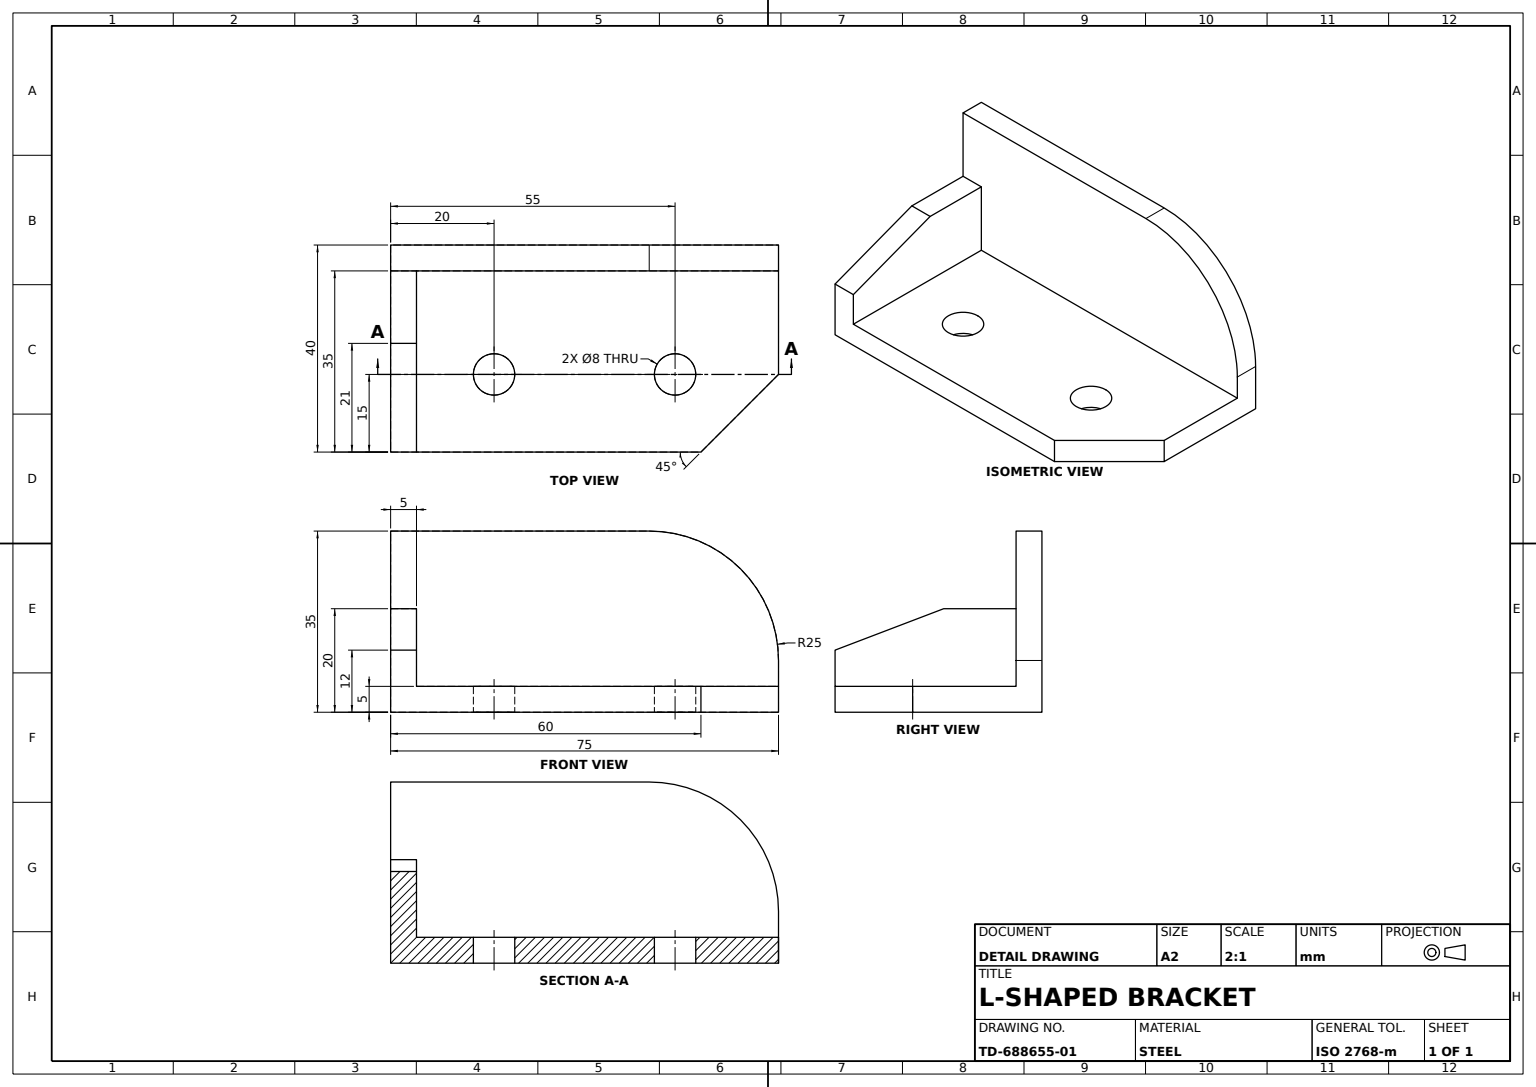
from build123d import *

# Parameters (mm, degrees)
BASE_PLATE_SKETCH_R           = 4
BASE_PLATE_DEPTH              = 5
SIDE_WALL_SKETCH_W            = 5
SIDE_WALL_SKETCH_H            = 40
SIDE_WALL_DEPTH               = 20
SIDE_WALL_TAPER_CUT_DEPTH     = 20
BACK_WALL_SKETCH_W            = 75
BACK_WALL_SKETCH_H            = 5
BACK_WALL_DEPTH               = 30
BACK_WALL_CORNER_RADIUS_DEPTH = 30


with BuildPart() as part:
    # Base Plate Sketch → Base Plate (new body)
    with BuildSketch(Plane(origin=(0, 0, 0), x_dir=(1, 0, 0), z_dir=(0, 1, 0))):
        Polygon((0, 0), (75, 0), (75, -25), (60, -40), (0, -40), align=None)
        with Locations(Location((20, -25, 0), (0, 0, 270))):
            Circle(BASE_PLATE_SKETCH_R, mode=Mode.SUBTRACT)
        with Locations(Location((55, -25, 0), (0, 0, 270))):
            Circle(BASE_PLATE_SKETCH_R, mode=Mode.SUBTRACT)
    extrude(amount=BASE_PLATE_DEPTH)

    # Side Wall Sketch → Side Wall (add)
    with BuildSketch(Plane(origin=(0, 5, 0), x_dir=(1, 0, 0), z_dir=(0, 1, 0))):
        with Locations((2.5, -20)):
            Rectangle(SIDE_WALL_SKETCH_W, SIDE_WALL_SKETCH_H)
    extrude(amount=SIDE_WALL_DEPTH)

    # Side Wall Taper Sketch → Side Wall Taper Cut (cut)
    with BuildSketch(Plane(origin=(5, 0, 0), x_dir=(0, 0, -1), z_dir=(1, 0, 0))):
        Polygon((-19, 20), (-40, 12), (-40, 25), (0, 25), (0, 20), align=None)
    extrude(amount=-SIDE_WALL_TAPER_CUT_DEPTH, mode=Mode.SUBTRACT)

    # Back Wall Sketch → Back Wall (add)
    with BuildSketch(Plane(origin=(0, 5, 0), x_dir=(1, 0, 0), z_dir=(0, 1, 0))):
        with Locations((37.5, -2.5)):
            Rectangle(BACK_WALL_SKETCH_W, BACK_WALL_SKETCH_H)
    extrude(amount=BACK_WALL_DEPTH)

    # Back Wall Corner Radius Sketch → Back Wall Corner Radius (cut)
    with BuildSketch(Plane.XY.offset(5)):
        with BuildLine():
            Line((50, 35), (75, 35))
            Line((75, 35), (75, 10))
            ThreePointArc((75, 10), (67.67766953, 27.67766953), (50, 35))
        make_face()
    extrude(amount=-BACK_WALL_CORNER_RADIUS_DEPTH, mode=Mode.SUBTRACT)


solid = part.part
